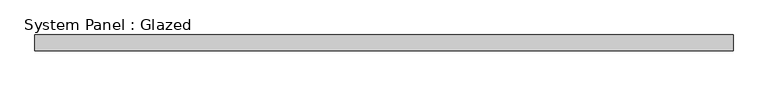
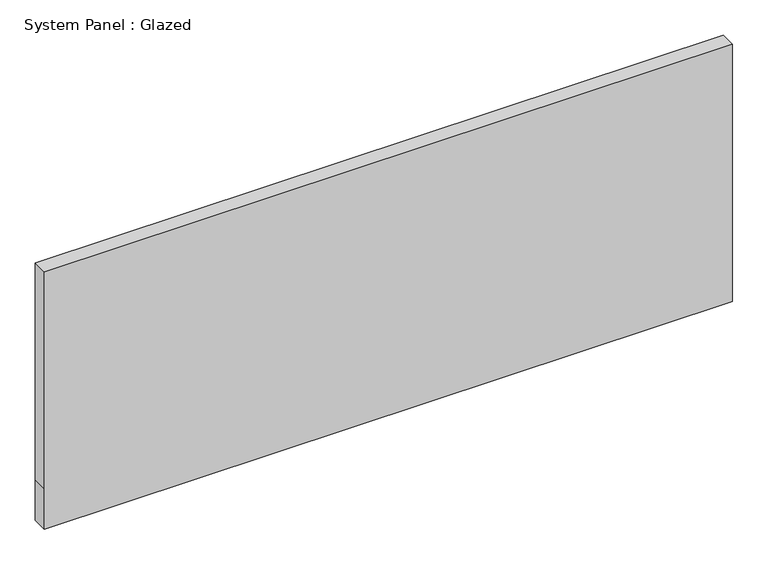
"""IFC4 building model written with IfcOpenShell, lengths in millimetres: plate geometry, System Panel : Glazed."""

from ifc_helpers import new_model, si_unit, frame, origin, place, context, project, spatial, polyline, outline, extrude, source, transform, mapped, element, save


def system_panel_glazed_d671f7fc(model_context):
    return source(origin(), model_context, "Body", "SweptSolid", [
        extrude(outline(polyline([(0.0, -561.975), (0.0, 561.975), (69.85, 561.975), (444.5, 561.975), (444.5, -561.975), (69.85, -561.975), (0.0, -561.975)])), frame((0.0, -44.45, 0.0), z_axis=(0.0, 1.0, 0.0), x_axis=(0.0, 0.0, 1.0)), (0.0, 0.0, 1.0), 25.4),
    ])


if __name__ == "__main__":
    model = new_model("IFC4")
    model_context = context("Model", 3, world=origin())
    ifc_project = project(units=[si_unit("LENGTHUNIT", "METRE", prefix="MILLI")], contexts=[model_context])
    site = spatial("IfcSite", under=ifc_project)
    building = spatial("IfcBuilding", under=site)
    placement = place(None, origin())
    system_panel_glazed_shape = system_panel_glazed_d671f7fc(model_context)
    element("IfcPlate", 1, ObjectType="System Panel : Glazed", at=placement, inside=building, context=model_context, shape_type="MappedRepresentation", body=[
        mapped(system_panel_glazed_shape, transform((0.0, 0.0, 0.0), x_axis=(1.0, 0.0, 0.0), y_axis=(0.0, 1.0, 0.0), z_axis=(0.0, 0.0, 1.0))),
    ])
    save(model, "model.ifc")

# Revit data of these elements
# Type "System Panel : Glazed"
#   Construction Type Id = "GSP4R"
#   Analytic Construction = "1/8 in Pilkington single glazing"
#   Visual Light Transmittance = 0.9
#   Solar Heat Gain Coefficient = 0.86
#   Heat Transfer Coefficient (U) = 1.18115 BTU/(h·ft²·°F)
#   Define Thermal Properties by = 1
# Element 1 (IfcPlate, "System Panel : Glazed")
#   Materials on its faces: "GARAGE PANEL"
# Materials
#   "GARAGE PANEL": class "Generic", colour RGB 120 120 120, transparency 0, Cost = 0
